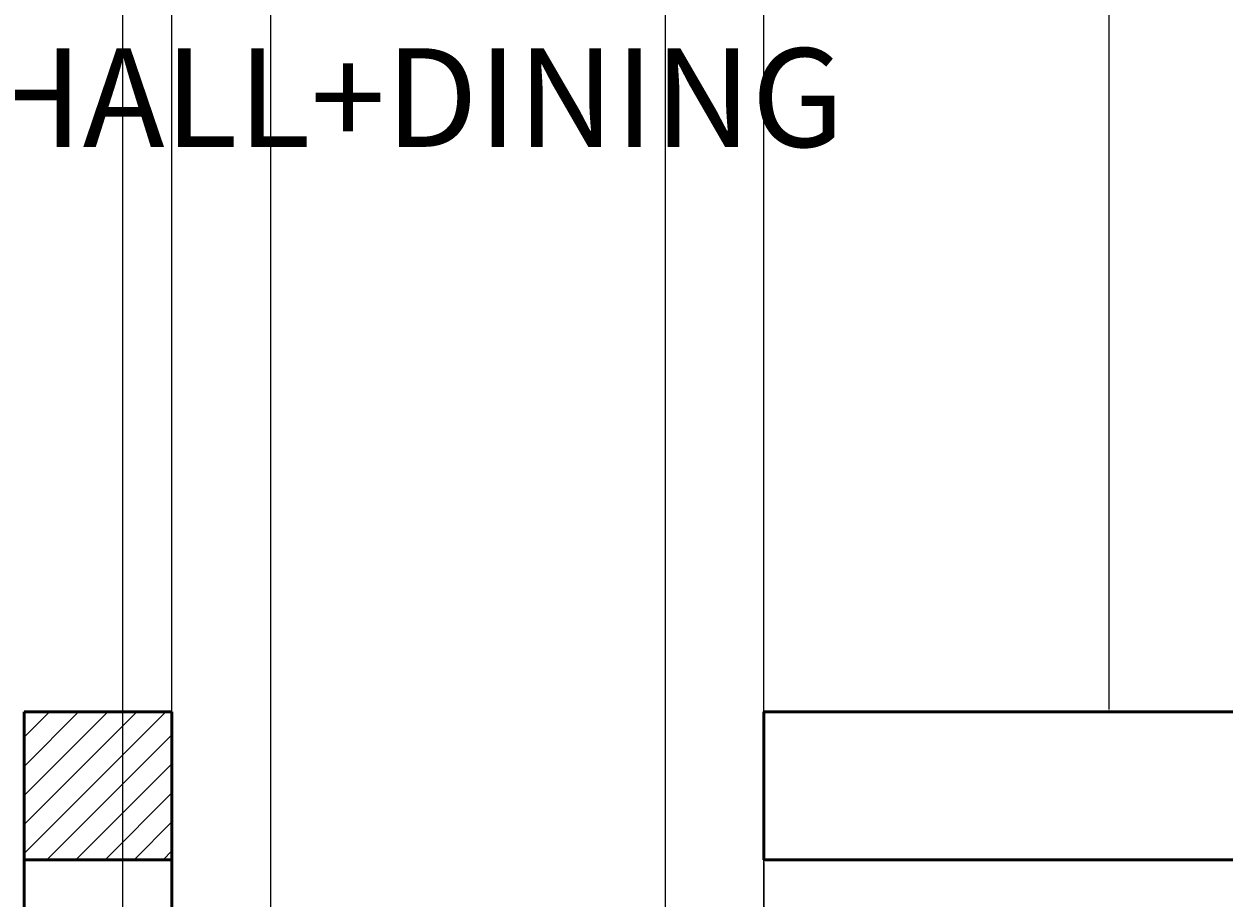
# Model space of a CAD drawing. Units: inches. Extents: x 0 to 281, y -535 to 46.
# Tile 4 of 22: x 150 to 223, y -275 to -222. Entities that reach past the tile are written whole.
import ezdxf

# ---------------------------------------------------------------- set-up
doc = ezdxf.new("R2010")
doc.units = ezdxf.units.IN
doc.header["$MEASUREMENT"] = 0
for name, color, linetype, lineweight in [('A-ANNO-DIMS', 2, 'Continuous', 18), ('A-AREA-IDEN', 7, 'Continuous', 25), ('A-COLS', 7, 'Continuous', 50), ('A-COLS-PATT', 152, 'Continuous', 13), ('A-WALL', 7, 'Continuous', 50)]:
    doc.layers.add(name, color=color, linetype=linetype, lineweight=lineweight)
doc.styles.get("Standard").update_dxf_attribs({"font": 'arial.ttf'})
doc.dimstyles.get("Standard").update_dxf_attribs({"dimtxt": 0.18, "dimasz": 0.18, "dimexe": 0.18, "dimexo": 0.0625, "dimgap": 0.09, "dimtad": 0, "dimtih": 1, "dimtoh": 1, "dimdec": 0, "dimzin": 0, "dimdsep": 46, "dimlunit": 3, "dimtxsty": 'Standard', "dimcen": 0.09, "dimadec": 0, "dimazin": 0, "dimtfac": 1, "dimtdec": 0, "dimtofl": 0, "dimtmove": 0, "dimatfit": 3, "dimfxl": 1, "dimtolj": 1, "dimtzin": 0, "dimarcsym": 0})

# ---------------------------------------------------------------- blocks, each defined once
blk = doc.blocks.new('*D6')
at = {"layer": 'A-ANNO-DIMS', "color": 0, "lineweight": -2, "transparency": 16777216}
for p, q in [((216.459, -131.591), (216.459, -194.308)), ((216.521, -131.411), (216.639, -131.411)), ((216.459, -263.231), (216.459, -200.513)), ((216.521, -263.411), (216.639, -263.411))]:
    blk.add_line(p, q, dxfattribs=at)
at = {"layer": 'A-ANNO-DIMS', "color": 0, "transparency": 16777216}
for points in [[(216.429, -131.591), (216.489, -131.591), (216.459, -131.411)], [(216.429, -263.231), (216.489, -263.231), (216.459, -263.411)]]:
    blk.add_solid(points, dxfattribs=at)
at = {"layer": 'Defpoints', "color": 0, "transparency": 16777216}
for p in [(216.459, -131.411), (216.459, -263.411), (216.459, -263.411)]:
    blk.add_point(p, dxfattribs=at)
at = {"layer": 'A-ANNO-DIMS', "color": 0, "transparency": 16777216, "insert": (216.459, -197.411), "char_height": 6, "attachment_point": 5}
blk.add_mtext("\\A1;11'", dxfattribs=at)
blk = doc.blocks.new('*D12')
at = {"layer": 'A-ANNO-DIMS', "color": 0, "lineweight": -2, "transparency": 16777216}
for p, q in [((195.459, -272.591), (195.459, -329.257)), ((195.521, -272.411), (195.639, -272.411)), ((195.459, -392.231), (195.459, -335.564)), ((195.521, -392.411), (195.639, -392.411))]:
    blk.add_line(p, q, dxfattribs=at)
at = {"layer": 'A-ANNO-DIMS', "color": 0, "transparency": 16777216}
for points in [[(195.429, -272.591), (195.489, -272.591), (195.459, -272.411)], [(195.429, -392.231), (195.489, -392.231), (195.459, -392.411)]]:
    blk.add_solid(points, dxfattribs=at)
at = {"layer": 'Defpoints', "color": 0, "transparency": 16777216}
for p in [(195.459, -272.411), (195.459, -392.411), (195.459, -392.411)]:
    blk.add_point(p, dxfattribs=at)
at = {"layer": 'A-ANNO-DIMS', "color": 0, "transparency": 16777216, "insert": (195.459, -332.411), "char_height": 6, "attachment_point": 5}
blk.add_mtext("\\A1;10'", dxfattribs=at)
blk = doc.blocks.new('*D41')
at = {"layer": 'A-ANNO-DIMS', "color": 0, "lineweight": -2, "transparency": 16777216}
for p, q in [((120.459, -131.473), (120.459, -535.041)), ((156.459, -131.473), (156.459, -535.041)), ((120.639, -534.861), (138.13, -534.861)), ((156.279, -534.861), (138.788, -534.861))]:
    blk.add_line(p, q, dxfattribs=at)
at = {"layer": 'A-ANNO-DIMS', "color": 0, "transparency": 16777216}
for points in [[(120.639, -534.831), (120.639, -534.891), (120.459, -534.861)], [(156.279, -534.831), (156.279, -534.891), (156.459, -534.861)]]:
    blk.add_solid(points, dxfattribs=at)
at = {"layer": 'Defpoints', "color": 0, "transparency": 16777216}
for p in [(120.459, -131.411), (156.459, -131.411), (156.459, -534.861)]:
    blk.add_point(p, dxfattribs=at)
at = {"layer": 'A-ANNO-DIMS', "color": 0, "transparency": 16777216, "insert": (138.459, -534.861), "char_height": 0.18, "attachment_point": 5}
blk.add_mtext('\\A1;3\'-0"', dxfattribs=at)
blk = doc.blocks.new('*D42')
at = {"layer": 'A-ANNO-DIMS', "color": 0, "lineweight": -2, "transparency": 16777216}
for p, q in [((165.459, -131.473), (165.459, -535.041)), ((189.459, -131.473), (189.459, -535.041)), ((165.639, -534.861), (177.128, -534.861)), ((189.279, -534.861), (177.79, -534.861))]:
    blk.add_line(p, q, dxfattribs=at)
at = {"layer": 'A-ANNO-DIMS', "color": 0, "transparency": 16777216}
for points in [[(165.639, -534.831), (165.639, -534.891), (165.459, -534.861)], [(189.279, -534.831), (189.279, -534.891), (189.459, -534.861)]]:
    blk.add_solid(points, dxfattribs=at)
at = {"layer": 'Defpoints', "color": 0, "transparency": 16777216}
for p in [(165.459, -131.411), (189.459, -131.411), (189.459, -534.861)]:
    blk.add_point(p, dxfattribs=at)
at = {"layer": 'A-ANNO-DIMS', "color": 0, "transparency": 16777216, "insert": (177.459, -534.861), "char_height": 0.18, "attachment_point": 5}
blk.add_mtext('\\A1;2\'-0"', dxfattribs=at)
blk = doc.blocks.new('*D46')
at = {"layer": 'A-ANNO-DIMS', "color": 0, "lineweight": -2, "transparency": 16777216}
for p, q in [((159.459, -263.348), (159.459, 46.219)), ((159.639, 46.039), (177.13, 46.039)), ((195.279, 46.039), (177.788, 46.039)), ((195.459, -263.348), (195.459, 46.219))]:
    blk.add_line(p, q, dxfattribs=at)
at = {"layer": 'A-ANNO-DIMS', "color": 0, "transparency": 16777216}
for points in [[(159.639, 46.069), (159.639, 46.009), (159.459, 46.039)], [(195.279, 46.069), (195.279, 46.009), (195.459, 46.039)]]:
    blk.add_solid(points, dxfattribs=at)
at = {"layer": 'Defpoints', "color": 0, "transparency": 16777216}
for p in [(195.459, 46.039), (159.459, -263.411), (195.459, -263.411)]:
    blk.add_point(p, dxfattribs=at)
at = {"layer": 'A-ANNO-DIMS', "color": 0, "transparency": 16777216, "insert": (177.459, 46.039), "char_height": 0.18, "attachment_point": 5}
blk.add_mtext('\\A1;3\'-0"', dxfattribs=at)
blk = doc.blocks.new('*D48')
at = {"layer": 'A-ANNO-DIMS', "color": 0, "lineweight": -2, "transparency": 16777216}
for p, q in [((159.459, -392.348), (159.459, 46.219)), ((159.639, 46.039), (177.13, 46.039)), ((195.279, 46.039), (177.788, 46.039)), ((195.459, -392.348), (195.459, 46.219))]:
    blk.add_line(p, q, dxfattribs=at)
at = {"layer": 'A-ANNO-DIMS', "color": 0, "transparency": 16777216}
for points in [[(159.639, 46.069), (159.639, 46.009), (159.459, 46.039)], [(195.279, 46.069), (195.279, 46.009), (195.459, 46.039)]]:
    blk.add_solid(points, dxfattribs=at)
at = {"layer": 'Defpoints', "color": 0, "transparency": 16777216}
for p in [(195.459, 46.039), (159.459, -392.411), (195.459, -392.411)]:
    blk.add_point(p, dxfattribs=at)
at = {"layer": 'A-ANNO-DIMS', "color": 0, "transparency": 16777216, "insert": (177.459, 46.039), "char_height": 0.18, "attachment_point": 5}
blk.add_mtext('\\A1;3\'-0"', dxfattribs=at)

msp = doc.modelspace()

# ---------------------------------------------------------------- hatches: boundary and pattern name
at = {"layer": 'A-COLS-PATT'}
h = msp.add_hatch(dxfattribs=at)
h.set_pattern_fill('ANSI31', color=256, scale=10)
h.paths.add_polyline_path([(165.459, -122.411), (156.459, -122.411), (156.459, -131.411), (165.459, -131.411)])
h.paths.add_polyline_path([(159.459, -263.411), (150.459, -263.411), (150.459, -272.411), (159.459, -272.411)])

# ---------------------------------------------------------------- linework, layer by layer
at = {"layer": 'A-COLS'}
for p, q in [((150.459, -263.411), (159.459, -263.411)), ((150.459, -272.411), (159.459, -272.411))]:
    msp.add_line(p, q, dxfattribs=at)
at = {"layer": 'A-WALL'}
for p, q in [((150.459, -263.411), (150.459, -401.411)), ((159.459, -263.411), (159.459, -401.411)), ((195.459, -272.411), (195.459, -263.411)), ((195.459, -263.411), (243.459, -263.411)), ((195.459, -272.411), (243.459, -272.411))]:
    msp.add_line(p, q, dxfattribs=at)

# ---------------------------------------------------------------- texts
at = {"layer": 'A-AREA-IDEN', "insert": (148.072, -223.048), "char_height": 6, "attachment_point": 1}
msp.add_mtext('HALL+DINING', dxfattribs=at)

# ---------------------------------------------------------------- dimensions: what is measured, and where the dimension line sits
at = {"layer": 'A-ANNO-DIMS'}
for base, p1, p2, picture, middle in [((195.459, 46.039), (159.459, -263.411), (195.459, -263.411), '*D46', (177.459, 46.039)), ((195.459, 46.039), (159.459, -392.411), (195.459, -392.411), '*D48', (177.459, 46.039)), ((156.459, -534.861), (120.459, -131.411), (156.459, -131.411), '*D41', (138.459, -534.861)), ((189.459, -534.861), (165.459, -131.411), (189.459, -131.411), '*D42', (177.459, -534.861))]:
    dim = msp.add_linear_dim(base=base, p1=p1, p2=p2, dimstyle='Standard', override={"dimdec": 1, "dimlfac": 1, "dimrnd": 0, "dimzin": 1, "dimdsep": 46, "dimlunit": 4, "dimfrac": 2}, dxfattribs=at)
    dim.commit()
    dim.dimension.update_dxf_attribs({"geometry": picture, "text_midpoint": middle})
for base, p1, p2, picture, middle in [((216.459, -263.411), (216.459, -131.411), (216.459, -263.411), '*D6', (216.459, -197.411)), ((195.459, -392.411), (195.459, -272.411), (195.459, -392.411), '*D12', (195.459, -332.411))]:
    dim = msp.add_linear_dim(base=base, p1=p1, p2=p2, angle=90, dimstyle='Standard', override={"dimtxt": 6, "dimclrd": 0, "dimclre": 0, "dimclrt": 0}, dxfattribs=at)
    dim.commit()
    dim.dimension.update_dxf_attribs({"geometry": picture, "text_midpoint": middle})

doc.saveas('drawing.dxf')
